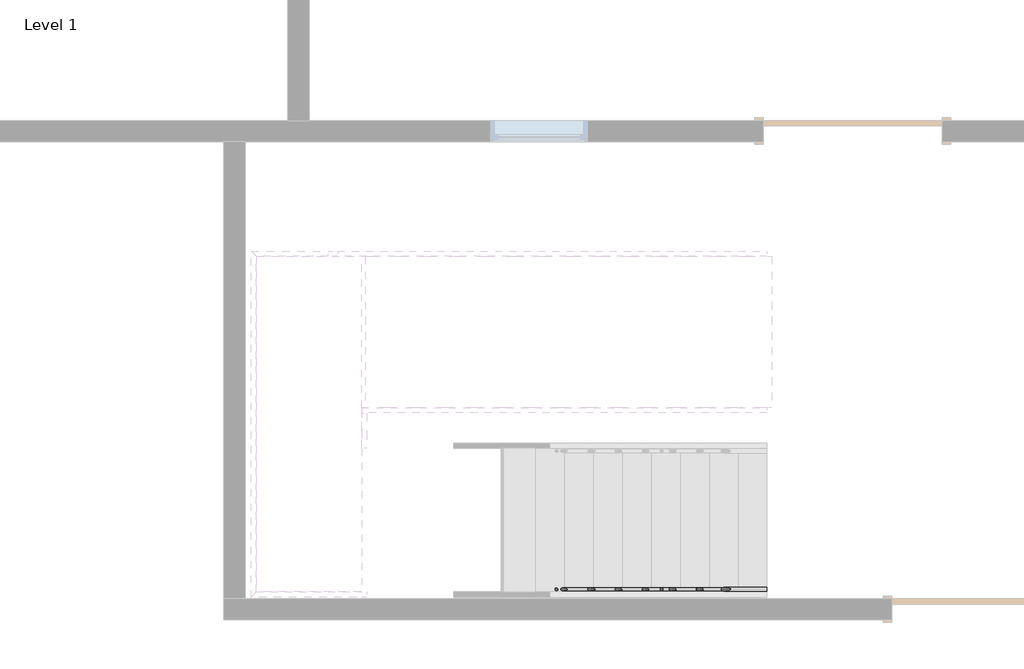
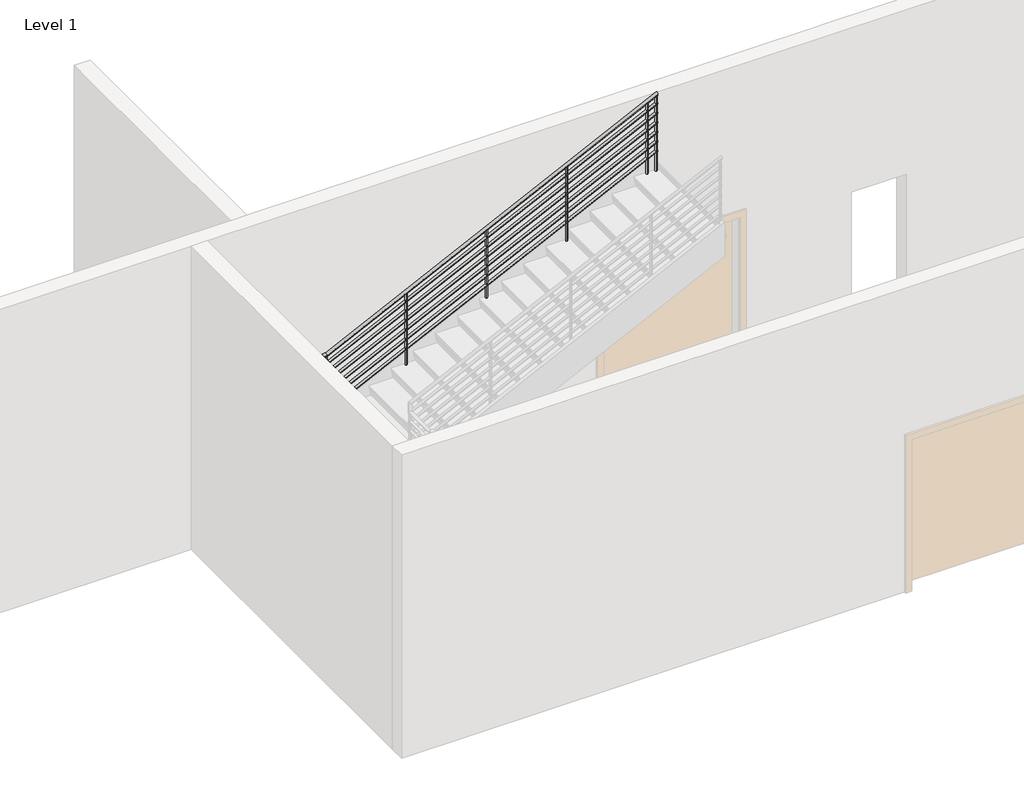
# One storey, part 3 of 4: 1 railing.
"""IFC4 building model written with IfcOpenShell, lengths in millimetres."""

from ifc_helpers import new_model, si_unit, point, frame, frame_2d, origin, place, context, project, spatial, circle_curve, ellipse_curve, trimmed, segment, composite_curve, outline, extrude, element, save
from ifc_brep_helpers import plane_surface, cylinder_surface, advanced_brep

model = new_model("IFC4")

# Units and contexts
model_context = context("Model", 3, world=origin())
ifc_project = project(units=[si_unit("LENGTHUNIT", "METRE", prefix="MILLI")], contexts=[model_context])

# Site, building, storey
site = spatial("IfcSite", under=ifc_project)
building = spatial("IfcBuilding", under=site)
storey = spatial("IfcBuildingStorey", under=building, Name="Level 1", Elevation=0.0)

# Railing
placement = place(None, origin())
element("IfcRailing", 1, ObjectType="900mm Pipe", at=placement, inside=storey, context=model_context, shape_type="SolidModel", body=[
    advanced_brep(
    [(3615.6033064, -1103.671626, 1011.1065202), (3615.6033064, -1143.671626, 1011.1065202), (-238.9894956, -1103.671626, 2880.0), (-238.9894956, -1143.671626, 2880.0), (-1189.0224748, -1103.671626, 2880.0), (-1229.0224748, -1143.671626, 2880.0), (-1189.0224748, 1993.0290713, 2880.0), (-1229.0224748, 2033.0290713, 2880.0), (-504.8038915, 1993.0290713, 2880.0), (-504.8038915, 2033.0290713, 2880.0), (3615.6033064, 1993.0290713, 4877.7731869), (3615.6033064, 2033.0290713, 4877.7731869)],
    [
        (0, 1, ellipse_curve(frame((3615.6033064, -1123.671626, 1011.1065202), z_axis=(1.0, 0.0, 0.0), x_axis=(0.0, 0.0, -1.0)), 22.2268131, 20.0)),
        (1, 0, ellipse_curve(frame((3615.6033064, -1123.671626, 1011.1065202), z_axis=(1.0, 0.0, 0.0), x_axis=(0.0, 0.0, -1.0)), 22.2268131, 20.0)),
        (0, 2),
        (2, 3, ellipse_curve(frame((-238.9894956, -1123.671626, 2880.0), z_axis=(0.9746317528164674, 0.0, -0.22381453572522994), x_axis=(-0.2238145357252298, 0.0, -0.9746317528164675)), 20.5205709, 20.0)),
        (3, 1),
        (3, 2, ellipse_curve(frame((-238.9894956, -1123.671626, 2880.0), z_axis=(0.9746317528164674, 0.0, -0.22381453572522994), x_axis=(-0.2238145357252298, 0.0, -0.9746317528164675)), 20.5205709, 20.0)),
        (2, 4),
        (4, 5, ellipse_curve(frame((-1209.0224748, -1123.671626, 2880.0), z_axis=(0.7071067811865449, -0.7071067811865501, 0.0), x_axis=(0.7071067811865501, 0.7071067811865449, 0.0)), 28.2842712, 20.0)),
        (5, 3),
        (5, 4, ellipse_curve(frame((-1209.0224748, -1123.671626, 2880.0), z_axis=(0.7071067811865449, -0.7071067811865501, 0.0), x_axis=(0.7071067811865501, 0.7071067811865449, 0.0)), 28.2842712, 20.0)),
        (4, 6),
        (6, 7, ellipse_curve(frame((-1209.0224748, 2013.0290713, 2880.0), z_axis=(-0.70710678118655, -0.7071067811865449, 0.0), x_axis=(0.7071067811865448, -0.7071067811865501, 0.0)), 28.2842712, 20.0)),
        (7, 5),
        (7, 6, ellipse_curve(frame((-1209.0224748, 2013.0290713, 2880.0), z_axis=(-0.70710678118655, -0.7071067811865449, 0.0), x_axis=(0.7071067811865448, -0.7071067811865501, 0.0)), 28.2842712, 20.0)),
        (6, 8),
        (8, 9, ellipse_curve(frame((-504.8038915, 2013.0290713, 2880.0), z_axis=(-0.9746317528164674, 0.0, -0.22381453572522989), x_axis=(-0.22381453572523038, 0.0, 0.9746317528164674)), 20.5205709, 20.0)),
        (9, 7),
        (9, 8, ellipse_curve(frame((-504.8038915, 2013.0290713, 2880.0), z_axis=(-0.9746317528164674, 0.0, -0.22381453572522989), x_axis=(-0.22381453572523038, 0.0, 0.9746317528164674)), 20.5205709, 20.0)),
        (10, 11, ellipse_curve(frame((3615.6033064, 2013.0290713, 4877.7731869), z_axis=(1.0, 0.0, 0.0), x_axis=(0.0, 0.0, -1.0)), 22.2268131, 20.0)),
        (11, 10, ellipse_curve(frame((3615.6033064, 2013.0290713, 4877.7731869), z_axis=(1.0, 0.0, 0.0), x_axis=(0.0, 0.0, -1.0)), 22.2268131, 20.0)),
        (8, 10),
        (11, 9),
    ],
    [
        plane_surface(frame((3615.6033064, -1123.671626, 1033.3333333), z_axis=(1.0, 0.0, 0.0), x_axis=(0.0, -1.0, 0.0))),
        cylinder_surface(frame((3606.8778363, -1123.671626, 1015.3370512), z_axis=(0.8998141071961996, 0.0, -0.4362735065193695), x_axis=(0.0, -1.0, 0.0)), 20.0),
        cylinder_surface(frame((-234.3966936, -1123.671626, 2880.0), z_axis=(1.0, 0.0, 0.0), x_axis=(0.0, -1.0, 0.0)), 20.0),
        cylinder_surface(frame((-1209.0224748, -1123.671626, 2880.0), z_axis=(0.0, -1.0, 0.0), x_axis=(-1.0, 0.0, 0.0)), 20.0),
        cylinder_surface(frame((-1209.0224748, 2013.0290713, 2880.0), z_axis=(-1.0, 0.0, 0.0), x_axis=(0.0, 1.0, 0.0)), 20.0),
        plane_surface(frame((3615.6033064, 2013.0290713, 4900.0), z_axis=(1.0, 0.0, 0.0), x_axis=(0.0, 1.0, 0.0))),
        cylinder_surface(frame((-500.6712235, 2013.0290713, 2882.0037179), z_axis=(-0.8998141071961996, 0.0, -0.4362735065193694), x_axis=(0.0, 1.0, 0.0)), 20.0),
    ],
    [
        (0, [[1, 2]]),
        (1, [[-1, 3, 4, 5]]),
        (1, [[-2, -5, 6, -3]]),
        (2, [[-4, 7, 8, 9]]),
        (2, [[-6, -9, 10, -7]]),
        (3, [[-8, 11, 12, 13]]),
        (3, [[-10, -13, 14, -11]]),
        (4, [[-12, 15, 16, 17]]),
        (4, [[-14, -17, 18, -15]]),
        (5, [[19, 20]]),
        (6, [[-16, 21, -20, 22]]),
        (6, [[-18, -22, -19, -21]]),
    ],
),
    advanced_brep(
    [(3615.6033064, -1108.671626, 891.6632235), (3615.6033064, -1138.671626, 891.6632235), (-237.8412951, -1108.671626, 2760.0), (-237.8412951, -1138.671626, 2760.0), (-1194.0224748, -1108.671626, 2760.0), (-1224.0224748, -1138.671626, 2760.0), (-1194.0224748, 1998.0290713, 2760.0), (-1224.0224748, 2028.0290713, 2760.0), (-505.952092, 1998.0290713, 2760.0), (-505.952092, 2028.0290713, 2760.0), (3615.6033064, 1998.0290713, 4758.3298902), (3615.6033064, 2028.0290713, 4758.3298902)],
    [
        (0, 1, ellipse_curve(frame((3615.6033064, -1123.671626, 891.6632235), z_axis=(1.0, 0.0, 0.0), x_axis=(0.0, 0.0, -1.0)), 16.6701098, 15.0)),
        (1, 0, ellipse_curve(frame((3615.6033064, -1123.671626, 891.6632235), z_axis=(1.0, 0.0, 0.0), x_axis=(0.0, 0.0, -1.0)), 16.6701098, 15.0)),
        (0, 2),
        (2, 3, ellipse_curve(frame((-237.8412951, -1123.671626, 2760.0), z_axis=(0.9746317528164674, 0.0, -0.22381453572522994), x_axis=(-0.2238145357252298, 0.0, -0.9746317528164675)), 15.3904282, 15.0)),
        (3, 1),
        (3, 2, ellipse_curve(frame((-237.8412951, -1123.671626, 2760.0), z_axis=(0.9746317528164674, 0.0, -0.22381453572522994), x_axis=(-0.2238145357252298, 0.0, -0.9746317528164675)), 15.3904282, 15.0)),
        (2, 4),
        (4, 5, ellipse_curve(frame((-1209.0224748, -1123.671626, 2760.0), z_axis=(0.7071067811865449, -0.7071067811865501, 0.0), x_axis=(0.7071067811865501, 0.7071067811865449, 0.0)), 21.2132034, 15.0)),
        (5, 3),
        (5, 4, ellipse_curve(frame((-1209.0224748, -1123.671626, 2760.0), z_axis=(0.7071067811865449, -0.7071067811865501, 0.0), x_axis=(0.7071067811865501, 0.7071067811865449, 0.0)), 21.2132034, 15.0)),
        (4, 6),
        (6, 7, ellipse_curve(frame((-1209.0224748, 2013.0290713, 2760.0), z_axis=(-0.70710678118655, -0.7071067811865449, 0.0), x_axis=(0.7071067811865448, -0.7071067811865501, 0.0)), 21.2132034, 15.0)),
        (7, 5),
        (7, 6, ellipse_curve(frame((-1209.0224748, 2013.0290713, 2760.0), z_axis=(-0.70710678118655, -0.7071067811865449, 0.0), x_axis=(0.7071067811865448, -0.7071067811865501, 0.0)), 21.2132034, 15.0)),
        (6, 8),
        (8, 9, ellipse_curve(frame((-505.952092, 2013.0290713, 2760.0), z_axis=(-0.9746317528164674, 0.0, -0.22381453572522989), x_axis=(-0.22381453572523038, 0.0, 0.9746317528164674)), 15.3904282, 15.0)),
        (9, 7),
        (9, 8, ellipse_curve(frame((-505.952092, 2013.0290713, 2760.0), z_axis=(-0.9746317528164674, 0.0, -0.22381453572522989), x_axis=(-0.22381453572523038, 0.0, 0.9746317528164674)), 15.3904282, 15.0)),
        (10, 11, ellipse_curve(frame((3615.6033064, 2013.0290713, 4758.3298902), z_axis=(1.0, 0.0, 0.0), x_axis=(0.0, 0.0, -1.0)), 16.6701098, 15.0)),
        (11, 10, ellipse_curve(frame((3615.6033064, 2013.0290713, 4758.3298902), z_axis=(1.0, 0.0, 0.0), x_axis=(0.0, 0.0, -1.0)), 16.6701098, 15.0)),
        (8, 10),
        (11, 9),
    ],
    [
        plane_surface(frame((3615.6033064, -1123.671626, 908.3333333), z_axis=(1.0, 0.0, 0.0), x_axis=(0.0, -1.0, 0.0))),
        cylinder_surface(frame((3609.0592038, -1123.671626, 894.8361217), z_axis=(0.8998141071961996, 0.0, -0.4362735065193695), x_axis=(0.0, -1.0, 0.0)), 15.0),
        cylinder_surface(frame((-234.3966936, -1123.671626, 2760.0), z_axis=(1.0, 0.0, 0.0), x_axis=(0.0, -1.0, 0.0)), 15.0),
        cylinder_surface(frame((-1209.0224748, -1123.671626, 2760.0), z_axis=(0.0, -1.0, 0.0), x_axis=(-1.0, 0.0, 0.0)), 15.0),
        cylinder_surface(frame((-1209.0224748, 2013.0290713, 2760.0), z_axis=(-1.0, 0.0, 0.0), x_axis=(0.0, 1.0, 0.0)), 15.0),
        plane_surface(frame((3615.6033064, 2013.0290713, 4775.0), z_axis=(1.0, 0.0, 0.0), x_axis=(0.0, 1.0, 0.0))),
        cylinder_surface(frame((-502.852591, 2013.0290713, 2761.5027884), z_axis=(-0.8998141071961996, 0.0, -0.4362735065193694), x_axis=(0.0, 1.0, 0.0)), 15.0),
    ],
    [
        (0, [[1, 2]]),
        (1, [[-1, 3, 4, 5]]),
        (1, [[-2, -5, 6, -3]]),
        (2, [[-4, 7, 8, 9]]),
        (2, [[-6, -9, 10, -7]]),
        (3, [[-8, 11, 12, 13]]),
        (3, [[-10, -13, 14, -11]]),
        (4, [[-12, 15, 16, 17]]),
        (4, [[-14, -17, 18, -15]]),
        (5, [[19, 20]]),
        (6, [[-16, 21, -20, 22]]),
        (6, [[-18, -22, -19, -21]]),
    ],
),
    advanced_brep(
    [(3615.6033064, -1108.671626, 766.6632235), (3615.6033064, -1138.671626, 766.6632235), (-237.8412951, -1108.671626, 2635.0), (-237.8412951, -1138.671626, 2635.0), (-1194.0224748, -1108.671626, 2635.0), (-1224.0224748, -1138.671626, 2635.0), (-1194.0224748, 1998.0290713, 2635.0), (-1224.0224748, 2028.0290713, 2635.0), (-505.952092, 1998.0290713, 2635.0), (-505.952092, 2028.0290713, 2635.0), (3615.6033064, 1998.0290713, 4633.3298902), (3615.6033064, 2028.0290713, 4633.3298902)],
    [
        (0, 1, ellipse_curve(frame((3615.6033064, -1123.671626, 766.6632235), z_axis=(1.0, 0.0, 0.0), x_axis=(0.0, 0.0, -1.0)), 16.6701098, 15.0)),
        (1, 0, ellipse_curve(frame((3615.6033064, -1123.671626, 766.6632235), z_axis=(1.0, 0.0, 0.0), x_axis=(0.0, 0.0, -1.0)), 16.6701098, 15.0)),
        (0, 2),
        (2, 3, ellipse_curve(frame((-237.8412951, -1123.671626, 2635.0), z_axis=(0.9746317528164674, 0.0, -0.22381453572522994), x_axis=(-0.2238145357252298, 0.0, -0.9746317528164675)), 15.3904282, 15.0)),
        (3, 1),
        (3, 2, ellipse_curve(frame((-237.8412951, -1123.671626, 2635.0), z_axis=(0.9746317528164674, 0.0, -0.22381453572522994), x_axis=(-0.2238145357252298, 0.0, -0.9746317528164675)), 15.3904282, 15.0)),
        (2, 4),
        (4, 5, ellipse_curve(frame((-1209.0224748, -1123.671626, 2635.0), z_axis=(0.7071067811865449, -0.7071067811865501, 0.0), x_axis=(0.7071067811865501, 0.7071067811865449, 0.0)), 21.2132034, 15.0)),
        (5, 3),
        (5, 4, ellipse_curve(frame((-1209.0224748, -1123.671626, 2635.0), z_axis=(0.7071067811865449, -0.7071067811865501, 0.0), x_axis=(0.7071067811865501, 0.7071067811865449, 0.0)), 21.2132034, 15.0)),
        (4, 6),
        (6, 7, ellipse_curve(frame((-1209.0224748, 2013.0290713, 2635.0), z_axis=(-0.70710678118655, -0.7071067811865449, 0.0), x_axis=(0.7071067811865448, -0.7071067811865501, 0.0)), 21.2132034, 15.0)),
        (7, 5),
        (7, 6, ellipse_curve(frame((-1209.0224748, 2013.0290713, 2635.0), z_axis=(-0.70710678118655, -0.7071067811865449, 0.0), x_axis=(0.7071067811865448, -0.7071067811865501, 0.0)), 21.2132034, 15.0)),
        (6, 8),
        (8, 9, ellipse_curve(frame((-505.952092, 2013.0290713, 2635.0), z_axis=(-0.9746317528164674, 0.0, -0.22381453572522989), x_axis=(-0.22381453572523038, 0.0, 0.9746317528164674)), 15.3904282, 15.0)),
        (9, 7),
        (9, 8, ellipse_curve(frame((-505.952092, 2013.0290713, 2635.0), z_axis=(-0.9746317528164674, 0.0, -0.22381453572522989), x_axis=(-0.22381453572523038, 0.0, 0.9746317528164674)), 15.3904282, 15.0)),
        (10, 11, ellipse_curve(frame((3615.6033064, 2013.0290713, 4633.3298902), z_axis=(1.0, 0.0, 0.0), x_axis=(0.0, 0.0, -1.0)), 16.6701098, 15.0)),
        (11, 10, ellipse_curve(frame((3615.6033064, 2013.0290713, 4633.3298902), z_axis=(1.0, 0.0, 0.0), x_axis=(0.0, 0.0, -1.0)), 16.6701098, 15.0)),
        (8, 10),
        (11, 9),
    ],
    [
        plane_surface(frame((3615.6033064, -1123.671626, 783.3333333), z_axis=(1.0, 0.0, 0.0), x_axis=(0.0, -1.0, 0.0))),
        cylinder_surface(frame((3609.0592038, -1123.671626, 769.8361217), z_axis=(0.8998141071961996, 0.0, -0.4362735065193695), x_axis=(0.0, -1.0, 0.0)), 15.0),
        cylinder_surface(frame((-234.3966936, -1123.671626, 2635.0), z_axis=(1.0, 0.0, 0.0), x_axis=(0.0, -1.0, 0.0)), 15.0),
        cylinder_surface(frame((-1209.0224748, -1123.671626, 2635.0), z_axis=(0.0, -1.0, 0.0), x_axis=(-1.0, 0.0, 0.0)), 15.0),
        cylinder_surface(frame((-1209.0224748, 2013.0290713, 2635.0), z_axis=(-1.0, 0.0, 0.0), x_axis=(0.0, 1.0, 0.0)), 15.0),
        plane_surface(frame((3615.6033064, 2013.0290713, 4650.0), z_axis=(1.0, 0.0, 0.0), x_axis=(0.0, 1.0, 0.0))),
        cylinder_surface(frame((-502.852591, 2013.0290713, 2636.5027884), z_axis=(-0.8998141071961996, 0.0, -0.4362735065193694), x_axis=(0.0, 1.0, 0.0)), 15.0),
    ],
    [
        (0, [[1, 2]]),
        (1, [[-1, 3, 4, 5]]),
        (1, [[-2, -5, 6, -3]]),
        (2, [[-4, 7, 8, 9]]),
        (2, [[-6, -9, 10, -7]]),
        (3, [[-8, 11, 12, 13]]),
        (3, [[-10, -13, 14, -11]]),
        (4, [[-12, 15, 16, 17]]),
        (4, [[-14, -17, 18, -15]]),
        (5, [[19, 20]]),
        (6, [[-16, 21, -20, 22]]),
        (6, [[-18, -22, -19, -21]]),
    ],
),
    advanced_brep(
    [(3615.6033064, -1108.671626, 641.6632235), (3615.6033064, -1138.671626, 641.6632235), (-237.8412951, -1108.671626, 2510.0), (-237.8412951, -1138.671626, 2510.0), (-1194.0224748, -1108.671626, 2510.0), (-1224.0224748, -1138.671626, 2510.0), (-1194.0224748, 1998.0290713, 2510.0), (-1224.0224748, 2028.0290713, 2510.0), (-505.952092, 1998.0290713, 2510.0), (-505.952092, 2028.0290713, 2510.0), (3615.6033064, 1998.0290713, 4508.3298902), (3615.6033064, 2028.0290713, 4508.3298902)],
    [
        (0, 1, ellipse_curve(frame((3615.6033064, -1123.671626, 641.6632235), z_axis=(1.0, 0.0, 0.0), x_axis=(0.0, 0.0, -1.0)), 16.6701098, 15.0)),
        (1, 0, ellipse_curve(frame((3615.6033064, -1123.671626, 641.6632235), z_axis=(1.0, 0.0, 0.0), x_axis=(0.0, 0.0, -1.0)), 16.6701098, 15.0)),
        (0, 2),
        (2, 3, ellipse_curve(frame((-237.8412951, -1123.671626, 2510.0), z_axis=(0.9746317528164674, 0.0, -0.2238145357252299), x_axis=(-0.22381453572522944, 0.0, -0.9746317528164676)), 15.3904282, 15.0)),
        (3, 1),
        (3, 2, ellipse_curve(frame((-237.8412951, -1123.671626, 2510.0), z_axis=(0.9746317528164674, 0.0, -0.2238145357252299), x_axis=(-0.22381453572522944, 0.0, -0.9746317528164676)), 15.3904282, 15.0)),
        (2, 4),
        (4, 5, ellipse_curve(frame((-1209.0224748, -1123.671626, 2510.0), z_axis=(0.7071067811865449, -0.7071067811865501, 0.0), x_axis=(0.7071067811865501, 0.7071067811865449, 0.0)), 21.2132034, 15.0)),
        (5, 3),
        (5, 4, ellipse_curve(frame((-1209.0224748, -1123.671626, 2510.0), z_axis=(0.7071067811865449, -0.7071067811865501, 0.0), x_axis=(0.7071067811865501, 0.7071067811865449, 0.0)), 21.2132034, 15.0)),
        (4, 6),
        (6, 7, ellipse_curve(frame((-1209.0224748, 2013.0290713, 2510.0), z_axis=(-0.70710678118655, -0.7071067811865449, 0.0), x_axis=(0.7071067811865448, -0.7071067811865501, 0.0)), 21.2132034, 15.0)),
        (7, 5),
        (7, 6, ellipse_curve(frame((-1209.0224748, 2013.0290713, 2510.0), z_axis=(-0.70710678118655, -0.7071067811865449, 0.0), x_axis=(0.7071067811865448, -0.7071067811865501, 0.0)), 21.2132034, 15.0)),
        (6, 8),
        (8, 9, ellipse_curve(frame((-505.952092, 2013.0290713, 2510.0), z_axis=(-0.9746317528164674, 0.0, -0.22381453572522994), x_axis=(-0.22381453572523038, 0.0, 0.9746317528164674)), 15.3904282, 15.0)),
        (9, 7),
        (9, 8, ellipse_curve(frame((-505.952092, 2013.0290713, 2510.0), z_axis=(-0.9746317528164674, 0.0, -0.22381453572522994), x_axis=(-0.22381453572523038, 0.0, 0.9746317528164674)), 15.3904282, 15.0)),
        (10, 11, ellipse_curve(frame((3615.6033064, 2013.0290713, 4508.3298902), z_axis=(1.0, 0.0, 0.0), x_axis=(0.0, 0.0, -1.0)), 16.6701098, 15.0)),
        (11, 10, ellipse_curve(frame((3615.6033064, 2013.0290713, 4508.3298902), z_axis=(1.0, 0.0, 0.0), x_axis=(0.0, 0.0, -1.0)), 16.6701098, 15.0)),
        (8, 10),
        (11, 9),
    ],
    [
        plane_surface(frame((3615.6033064, -1123.671626, 658.3333333), z_axis=(1.0, 0.0, 0.0), x_axis=(0.0, -1.0, 0.0))),
        cylinder_surface(frame((3609.0592038, -1123.671626, 644.8361217), z_axis=(0.8998141071961997, 0.0, -0.4362735065193694), x_axis=(0.0, -1.0, 0.0)), 15.0),
        cylinder_surface(frame((-234.3966936, -1123.671626, 2510.0), z_axis=(1.0, 0.0, 0.0), x_axis=(0.0, -1.0, 0.0)), 15.0),
        cylinder_surface(frame((-1209.0224748, -1123.671626, 2510.0), z_axis=(0.0, -1.0, 0.0), x_axis=(-1.0, 0.0, 0.0)), 15.0),
        cylinder_surface(frame((-1209.0224748, 2013.0290713, 2510.0), z_axis=(-1.0, 0.0, 0.0), x_axis=(0.0, 1.0, 0.0)), 15.0),
        plane_surface(frame((3615.6033064, 2013.0290713, 4525.0), z_axis=(1.0, 0.0, 0.0), x_axis=(0.0, 1.0, 0.0))),
        cylinder_surface(frame((-502.852591, 2013.0290713, 2511.5027884), z_axis=(-0.8998141071961996, 0.0, -0.43627350651936947), x_axis=(0.0, 1.0, 0.0)), 15.0),
    ],
    [
        (0, [[1, 2]]),
        (1, [[-1, 3, 4, 5]]),
        (1, [[-2, -5, 6, -3]]),
        (2, [[-4, 7, 8, 9]]),
        (2, [[-6, -9, 10, -7]]),
        (3, [[-8, 11, 12, 13]]),
        (3, [[-10, -13, 14, -11]]),
        (4, [[-12, 15, 16, 17]]),
        (4, [[-14, -17, 18, -15]]),
        (5, [[19, 20]]),
        (6, [[-16, 21, -20, 22]]),
        (6, [[-18, -22, -19, -21]]),
    ],
),
    advanced_brep(
    [(3615.6033064, -1108.671626, 516.6632235), (3615.6033064, -1138.671626, 516.6632235), (-237.8412951, -1108.671626, 2385.0), (-237.8412951, -1138.671626, 2385.0), (-1194.0224748, -1108.671626, 2385.0), (-1224.0224748, -1138.671626, 2385.0), (-1194.0224748, 1998.0290713, 2385.0), (-1224.0224748, 2028.0290713, 2385.0), (-505.952092, 1998.0290713, 2385.0), (-505.952092, 2028.0290713, 2385.0), (3615.6033064, 1998.0290713, 4383.3298902), (3615.6033064, 2028.0290713, 4383.3298902)],
    [
        (0, 1, ellipse_curve(frame((3615.6033064, -1123.671626, 516.6632235), z_axis=(1.0, 0.0, 0.0), x_axis=(0.0, 0.0, -1.0)), 16.6701098, 15.0)),
        (1, 0, ellipse_curve(frame((3615.6033064, -1123.671626, 516.6632235), z_axis=(1.0, 0.0, 0.0), x_axis=(0.0, 0.0, -1.0)), 16.6701098, 15.0)),
        (0, 2),
        (2, 3, ellipse_curve(frame((-237.8412951, -1123.671626, 2385.0), z_axis=(0.9746317528164674, 0.0, -0.22381453572522994), x_axis=(-0.2238145357252298, 0.0, -0.9746317528164675)), 15.3904282, 15.0)),
        (3, 1),
        (3, 2, ellipse_curve(frame((-237.8412951, -1123.671626, 2385.0), z_axis=(0.9746317528164674, 0.0, -0.22381453572522994), x_axis=(-0.2238145357252298, 0.0, -0.9746317528164675)), 15.3904282, 15.0)),
        (2, 4),
        (4, 5, ellipse_curve(frame((-1209.0224748, -1123.671626, 2385.0), z_axis=(0.7071067811865449, -0.7071067811865501, 0.0), x_axis=(0.7071067811865501, 0.7071067811865449, 0.0)), 21.2132034, 15.0)),
        (5, 3),
        (5, 4, ellipse_curve(frame((-1209.0224748, -1123.671626, 2385.0), z_axis=(0.7071067811865449, -0.7071067811865501, 0.0), x_axis=(0.7071067811865501, 0.7071067811865449, 0.0)), 21.2132034, 15.0)),
        (4, 6),
        (6, 7, ellipse_curve(frame((-1209.0224748, 2013.0290713, 2385.0), z_axis=(-0.70710678118655, -0.7071067811865449, 0.0), x_axis=(0.7071067811865448, -0.7071067811865501, 0.0)), 21.2132034, 15.0)),
        (7, 5),
        (7, 6, ellipse_curve(frame((-1209.0224748, 2013.0290713, 2385.0), z_axis=(-0.70710678118655, -0.7071067811865449, 0.0), x_axis=(0.7071067811865448, -0.7071067811865501, 0.0)), 21.2132034, 15.0)),
        (6, 8),
        (8, 9, ellipse_curve(frame((-505.952092, 2013.0290713, 2385.0), z_axis=(-0.9746317528164674, 0.0, -0.22381453572522989), x_axis=(-0.22381453572523038, 0.0, 0.9746317528164674)), 15.3904282, 15.0)),
        (9, 7),
        (9, 8, ellipse_curve(frame((-505.952092, 2013.0290713, 2385.0), z_axis=(-0.9746317528164674, 0.0, -0.22381453572522989), x_axis=(-0.22381453572523038, 0.0, 0.9746317528164674)), 15.3904282, 15.0)),
        (10, 11, ellipse_curve(frame((3615.6033064, 2013.0290713, 4383.3298902), z_axis=(1.0, 0.0, 0.0), x_axis=(0.0, 0.0, -1.0)), 16.6701098, 15.0)),
        (11, 10, ellipse_curve(frame((3615.6033064, 2013.0290713, 4383.3298902), z_axis=(1.0, 0.0, 0.0), x_axis=(0.0, 0.0, -1.0)), 16.6701098, 15.0)),
        (8, 10),
        (11, 9),
    ],
    [
        plane_surface(frame((3615.6033064, -1123.671626, 533.3333333), z_axis=(1.0, 0.0, 0.0), x_axis=(0.0, -1.0, 0.0))),
        cylinder_surface(frame((3609.0592038, -1123.671626, 519.8361217), z_axis=(0.8998141071961996, 0.0, -0.4362735065193695), x_axis=(0.0, -1.0, 0.0)), 15.0),
        cylinder_surface(frame((-234.3966936, -1123.671626, 2385.0), z_axis=(1.0, 0.0, 0.0), x_axis=(0.0, -1.0, 0.0)), 15.0),
        cylinder_surface(frame((-1209.0224748, -1123.671626, 2385.0), z_axis=(0.0, -1.0, 0.0), x_axis=(-1.0, 0.0, 0.0)), 15.0),
        cylinder_surface(frame((-1209.0224748, 2013.0290713, 2385.0), z_axis=(-1.0, 0.0, 0.0), x_axis=(0.0, 1.0, 0.0)), 15.0),
        plane_surface(frame((3615.6033064, 2013.0290713, 4400.0), z_axis=(1.0, 0.0, 0.0), x_axis=(0.0, 1.0, 0.0))),
        cylinder_surface(frame((-502.852591, 2013.0290713, 2386.5027884), z_axis=(-0.8998141071961996, 0.0, -0.4362735065193694), x_axis=(0.0, 1.0, 0.0)), 15.0),
    ],
    [
        (0, [[1, 2]]),
        (1, [[-1, 3, 4, 5]]),
        (1, [[-2, -5, 6, -3]]),
        (2, [[-4, 7, 8, 9]]),
        (2, [[-6, -9, 10, -7]]),
        (3, [[-8, 11, 12, 13]]),
        (3, [[-10, -13, 14, -11]]),
        (4, [[-12, 15, 16, 17]]),
        (4, [[-14, -17, 18, -15]]),
        (5, [[19, 20]]),
        (6, [[-16, 21, -20, 22]]),
        (6, [[-18, -22, -19, -21]]),
    ],
),
    advanced_brep(
    [(3615.6033064, -1108.671626, 391.6632235), (3615.6033064, -1138.671626, 391.6632235), (-237.8412951, -1108.671626, 2260.0), (-237.8412951, -1138.671626, 2260.0), (-1194.0224748, -1108.671626, 2260.0), (-1224.0224748, -1138.671626, 2260.0), (-1194.0224748, 1998.0290713, 2260.0), (-1224.0224748, 2028.0290713, 2260.0), (-505.952092, 1998.0290713, 2260.0), (-505.952092, 2028.0290713, 2260.0), (3615.6033064, 1998.0290713, 4258.3298902), (3615.6033064, 2028.0290713, 4258.3298902)],
    [
        (0, 1, ellipse_curve(frame((3615.6033064, -1123.671626, 391.6632235), z_axis=(1.0, 0.0, 0.0), x_axis=(0.0, 0.0, -1.0)), 16.6701098, 15.0)),
        (1, 0, ellipse_curve(frame((3615.6033064, -1123.671626, 391.6632235), z_axis=(1.0, 0.0, 0.0), x_axis=(0.0, 0.0, -1.0)), 16.6701098, 15.0)),
        (0, 2),
        (2, 3, ellipse_curve(frame((-237.8412951, -1123.671626, 2260.0), z_axis=(0.9746317528164674, 0.0, -0.22381453572522994), x_axis=(-0.2238145357252298, 0.0, -0.9746317528164675)), 15.3904282, 15.0)),
        (3, 1),
        (3, 2, ellipse_curve(frame((-237.8412951, -1123.671626, 2260.0), z_axis=(0.9746317528164674, 0.0, -0.22381453572522994), x_axis=(-0.2238145357252298, 0.0, -0.9746317528164675)), 15.3904282, 15.0)),
        (2, 4),
        (4, 5, ellipse_curve(frame((-1209.0224748, -1123.671626, 2260.0), z_axis=(0.7071067811865449, -0.7071067811865501, 0.0), x_axis=(0.7071067811865501, 0.7071067811865449, 0.0)), 21.2132034, 15.0)),
        (5, 3),
        (5, 4, ellipse_curve(frame((-1209.0224748, -1123.671626, 2260.0), z_axis=(0.7071067811865449, -0.7071067811865501, 0.0), x_axis=(0.7071067811865501, 0.7071067811865449, 0.0)), 21.2132034, 15.0)),
        (4, 6),
        (6, 7, ellipse_curve(frame((-1209.0224748, 2013.0290713, 2260.0), z_axis=(-0.70710678118655, -0.7071067811865449, 0.0), x_axis=(0.7071067811865448, -0.7071067811865501, 0.0)), 21.2132034, 15.0)),
        (7, 5),
        (7, 6, ellipse_curve(frame((-1209.0224748, 2013.0290713, 2260.0), z_axis=(-0.70710678118655, -0.7071067811865449, 0.0), x_axis=(0.7071067811865448, -0.7071067811865501, 0.0)), 21.2132034, 15.0)),
        (6, 8),
        (8, 9, ellipse_curve(frame((-505.952092, 2013.0290713, 2260.0), z_axis=(-0.9746317528164674, 0.0, -0.2238145357252299), x_axis=(-0.22381453572523033, 0.0, 0.9746317528164674)), 15.3904282, 15.0)),
        (9, 7),
        (9, 8, ellipse_curve(frame((-505.952092, 2013.0290713, 2260.0), z_axis=(-0.9746317528164674, 0.0, -0.2238145357252299), x_axis=(-0.22381453572523033, 0.0, 0.9746317528164674)), 15.3904282, 15.0)),
        (10, 11, ellipse_curve(frame((3615.6033064, 2013.0290713, 4258.3298902), z_axis=(1.0, 0.0, 0.0), x_axis=(0.0, 0.0, -1.0)), 16.6701098, 15.0)),
        (11, 10, ellipse_curve(frame((3615.6033064, 2013.0290713, 4258.3298902), z_axis=(1.0, 0.0, 0.0), x_axis=(0.0, 0.0, -1.0)), 16.6701098, 15.0)),
        (8, 10),
        (11, 9),
    ],
    [
        plane_surface(frame((3615.6033064, -1123.671626, 408.3333333), z_axis=(1.0, 0.0, 0.0), x_axis=(0.0, -1.0, 0.0))),
        cylinder_surface(frame((3609.0592038, -1123.671626, 394.8361217), z_axis=(0.8998141071961996, 0.0, -0.4362735065193695), x_axis=(0.0, -1.0, 0.0)), 15.0),
        cylinder_surface(frame((-234.3966936, -1123.671626, 2260.0), z_axis=(1.0, 0.0, 0.0), x_axis=(0.0, -1.0, 0.0)), 15.0),
        cylinder_surface(frame((-1209.0224748, -1123.671626, 2260.0), z_axis=(0.0, -1.0, 0.0), x_axis=(-1.0, 0.0, 0.0)), 15.0),
        cylinder_surface(frame((-1209.0224748, 2013.0290713, 2260.0), z_axis=(-1.0, 0.0, 0.0), x_axis=(0.0, 1.0, 0.0)), 15.0),
        plane_surface(frame((3615.6033064, 2013.0290713, 4275.0), z_axis=(1.0, 0.0, 0.0), x_axis=(0.0, 1.0, 0.0))),
        cylinder_surface(frame((-502.852591, 2013.0290713, 2261.5027884), z_axis=(-0.8998141071961996, 0.0, -0.43627350651936947), x_axis=(0.0, 1.0, 0.0)), 15.0),
    ],
    [
        (0, [[1, 2]]),
        (1, [[-1, 3, 4, 5]]),
        (1, [[-2, -5, 6, -3]]),
        (2, [[-4, 7, 8, 9]]),
        (2, [[-6, -9, 10, -7]]),
        (3, [[-8, 11, 12, 13]]),
        (3, [[-10, -13, 14, -11]]),
        (4, [[-12, 15, 16, 17]]),
        (4, [[-14, -17, 18, -15]]),
        (5, [[19, 20]]),
        (6, [[-16, 21, -20, 22]]),
        (6, [[-18, -22, -19, -21]]),
    ],
),
    advanced_brep(
    [(3615.6033064, -1108.671626, 266.6632235), (3615.6033064, -1138.671626, 266.6632235), (-237.8412951, -1108.671626, 2135.0), (-237.8412951, -1138.671626, 2135.0), (-1194.0224748, -1108.671626, 2135.0), (-1224.0224748, -1138.671626, 2135.0), (-1194.0224748, 1998.0290713, 2135.0), (-1224.0224748, 2028.0290713, 2135.0), (-505.952092, 1998.0290713, 2135.0), (-505.952092, 2028.0290713, 2135.0), (3615.6033064, 1998.0290713, 4133.3298902), (3615.6033064, 2028.0290713, 4133.3298902)],
    [
        (0, 1, ellipse_curve(frame((3615.6033064, -1123.671626, 266.6632235), z_axis=(1.0, 0.0, 0.0), x_axis=(0.0, 0.0, -1.0)), 16.6701098, 15.0)),
        (1, 0, ellipse_curve(frame((3615.6033064, -1123.671626, 266.6632235), z_axis=(1.0, 0.0, 0.0), x_axis=(0.0, 0.0, -1.0)), 16.6701098, 15.0)),
        (0, 2),
        (2, 3, ellipse_curve(frame((-237.8412951, -1123.671626, 2135.0), z_axis=(0.9746317528164674, 0.0, -0.22381453572522994), x_axis=(-0.2238145357252298, 0.0, -0.9746317528164675)), 15.3904282, 15.0)),
        (3, 1),
        (3, 2, ellipse_curve(frame((-237.8412951, -1123.671626, 2135.0), z_axis=(0.9746317528164674, 0.0, -0.22381453572522994), x_axis=(-0.2238145357252298, 0.0, -0.9746317528164675)), 15.3904282, 15.0)),
        (2, 4),
        (4, 5, ellipse_curve(frame((-1209.0224748, -1123.671626, 2135.0), z_axis=(0.7071067811865449, -0.7071067811865501, 0.0), x_axis=(0.7071067811865501, 0.7071067811865449, 0.0)), 21.2132034, 15.0)),
        (5, 3),
        (5, 4, ellipse_curve(frame((-1209.0224748, -1123.671626, 2135.0), z_axis=(0.7071067811865449, -0.7071067811865501, 0.0), x_axis=(0.7071067811865501, 0.7071067811865449, 0.0)), 21.2132034, 15.0)),
        (4, 6),
        (6, 7, ellipse_curve(frame((-1209.0224748, 2013.0290713, 2135.0), z_axis=(-0.70710678118655, -0.7071067811865449, 0.0), x_axis=(0.7071067811865448, -0.7071067811865501, 0.0)), 21.2132034, 15.0)),
        (7, 5),
        (7, 6, ellipse_curve(frame((-1209.0224748, 2013.0290713, 2135.0), z_axis=(-0.70710678118655, -0.7071067811865449, 0.0), x_axis=(0.7071067811865448, -0.7071067811865501, 0.0)), 21.2132034, 15.0)),
        (6, 8),
        (8, 9, ellipse_curve(frame((-505.952092, 2013.0290713, 2135.0), z_axis=(-0.9746317528164674, 0.0, -0.22381453572522989), x_axis=(-0.22381453572523038, 0.0, 0.9746317528164674)), 15.3904282, 15.0)),
        (9, 7),
        (9, 8, ellipse_curve(frame((-505.952092, 2013.0290713, 2135.0), z_axis=(-0.9746317528164674, 0.0, -0.22381453572522989), x_axis=(-0.22381453572523038, 0.0, 0.9746317528164674)), 15.3904282, 15.0)),
        (10, 11, ellipse_curve(frame((3615.6033064, 2013.0290713, 4133.3298902), z_axis=(1.0, 0.0, 0.0), x_axis=(0.0, 0.0, -1.0)), 16.6701098, 15.0)),
        (11, 10, ellipse_curve(frame((3615.6033064, 2013.0290713, 4133.3298902), z_axis=(1.0, 0.0, 0.0), x_axis=(0.0, 0.0, -1.0)), 16.6701098, 15.0)),
        (8, 10),
        (11, 9),
    ],
    [
        plane_surface(frame((3615.6033064, -1123.671626, 283.3333333), z_axis=(1.0, 0.0, 0.0), x_axis=(0.0, -1.0, 0.0))),
        cylinder_surface(frame((3609.0592038, -1123.671626, 269.8361217), z_axis=(0.8998141071961996, 0.0, -0.4362735065193695), x_axis=(0.0, -1.0, 0.0)), 15.0),
        cylinder_surface(frame((-234.3966936, -1123.671626, 2135.0), z_axis=(1.0, 0.0, 0.0), x_axis=(0.0, -1.0, 0.0)), 15.0),
        cylinder_surface(frame((-1209.0224748, -1123.671626, 2135.0), z_axis=(0.0, -1.0, 0.0), x_axis=(-1.0, 0.0, 0.0)), 15.0),
        cylinder_surface(frame((-1209.0224748, 2013.0290713, 2135.0), z_axis=(-1.0, 0.0, 0.0), x_axis=(0.0, 1.0, 0.0)), 15.0),
        plane_surface(frame((3615.6033064, 2013.0290713, 4150.0), z_axis=(1.0, 0.0, 0.0), x_axis=(0.0, 1.0, 0.0))),
        cylinder_surface(frame((-502.852591, 2013.0290713, 2136.5027884), z_axis=(-0.8998141071961996, 0.0, -0.4362735065193694), x_axis=(0.0, 1.0, 0.0)), 15.0),
    ],
    [
        (0, [[1, 2]]),
        (1, [[-1, 3, 4, 5]]),
        (1, [[-2, -5, 6, -3]]),
        (2, [[-4, 7, 8, 9]]),
        (2, [[-6, -9, 10, -7]]),
        (3, [[-8, 11, 12, 13]]),
        (3, [[-10, -13, 14, -11]]),
        (4, [[-12, 15, 16, 17]]),
        (4, [[-14, -17, 18, -15]]),
        (5, [[19, 20]]),
        (6, [[-16, 21, -20, 22]]),
        (6, [[-18, -22, -19, -21]]),
    ],
),
    advanced_brep(
    [(3490.6033064, 2025.5290713, 4794.9403132), (3490.6033064, 2000.5290713, 4794.9403132), (3490.6033064, 2000.5290713, 3866.6666667), (3490.6033064, 2025.5290713, 3866.6666667)],
    [
        (0, 1, ellipse_curve(frame((3490.6033064, 2013.0290713, 4794.9403132), z_axis=(0.43627350651937075, 0.0, -0.899814107196199), x_axis=(0.8998141071961991, 0.0, 0.43627350651937047)), 13.8917582, 12.5)),
        (1, 2),
        (2, 3, circle_curve(frame((3490.6033064, 2013.0290713, 3866.6666667), z_axis=(0.0, 0.0, 1.0), x_axis=(0.0, -1.0, 0.0)), 12.5)),
        (3, 0),
        (3, 2, circle_curve(frame((3490.6033064, 2013.0290713, 3866.6666667), z_axis=(0.0, 0.0, 1.0), x_axis=(0.0, -1.0, 0.0)), 12.5)),
        (1, 0, ellipse_curve(frame((3490.6033064, 2013.0290713, 4794.9403132), z_axis=(0.43627350651937075, 0.0, -0.899814107196199), x_axis=(0.8998141071961991, 0.0, 0.43627350651937047)), 13.8917582, 12.5)),
    ],
    [
        cylinder_surface(frame((3490.6033064, 2013.0290713, 3766.6666667), z_axis=(0.0, 0.0, 1.0), x_axis=(0.0, -1.0, 0.0)), 12.5),
        plane_surface(frame((3515.6033064, 1988.0290713, 4807.0615253), z_axis=(-0.43627350651937075, 0.0, 0.899814107196199), x_axis=(0.0, 1.0, 0.0))),
        plane_surface(frame((3465.6033064, 1988.0290713, 3866.6666667), z_axis=(0.0, 0.0, -1.0), x_axis=(0.0, 1.0, 0.0))),
    ],
    [
        (0, [[1, 2, 3, 4]]),
        (0, [[5, -2, 6, -4]]),
        (1, [[-6, -1]]),
        (2, [[-5, -3]]),
    ],
),
    advanced_brep(
    [(2490.6033064, 2025.5290713, 4310.0918283), (2490.6033064, 2000.5290713, 4310.0918283), (2490.6033064, 2000.5290713, 3333.3333333), (2490.6033064, 2025.5290713, 3333.3333333)],
    [
        (0, 1, ellipse_curve(frame((2490.6033064, 2013.0290713, 4310.0918283), z_axis=(0.43627350651937075, 0.0, -0.899814107196199), x_axis=(0.8998141071961991, 0.0, 0.43627350651937047)), 13.8917582, 12.5)),
        (1, 2),
        (2, 3, circle_curve(frame((2490.6033064, 2013.0290713, 3333.3333333), z_axis=(0.0, 0.0, 1.0), x_axis=(0.0, -1.0, 0.0)), 12.5)),
        (3, 0),
        (3, 2, circle_curve(frame((2490.6033064, 2013.0290713, 3333.3333333), z_axis=(0.0, 0.0, 1.0), x_axis=(0.0, -1.0, 0.0)), 12.5)),
        (1, 0, ellipse_curve(frame((2490.6033064, 2013.0290713, 4310.0918283), z_axis=(0.43627350651937075, 0.0, -0.899814107196199), x_axis=(0.8998141071961991, 0.0, 0.43627350651937047)), 13.8917582, 12.5)),
    ],
    [
        cylinder_surface(frame((2490.6033064, 2013.0290713, 3233.3333333), z_axis=(0.0, 0.0, 1.0), x_axis=(0.0, -1.0, 0.0)), 12.5),
        plane_surface(frame((2515.6033064, 1988.0290713, 4322.2130404), z_axis=(-0.43627350651937075, 0.0, 0.899814107196199), x_axis=(0.0, 1.0, 0.0))),
        plane_surface(frame((2465.6033064, 1988.0290713, 3333.3333333), z_axis=(0.0, 0.0, -1.0), x_axis=(0.0, 1.0, 0.0))),
    ],
    [
        (0, [[1, 2, 3, 4]]),
        (0, [[5, -2, 6, -4]]),
        (1, [[-6, -1]]),
        (2, [[-5, -3]]),
    ],
),
    advanced_brep(
    [(1490.6033064, 2025.5290713, 3825.2433435), (1490.6033064, 2000.5290713, 3825.2433435), (1490.6033064, 2000.5290713, 2933.3333333), (1490.6033064, 2025.5290713, 2933.3333333)],
    [
        (0, 1, ellipse_curve(frame((1490.6033064, 2013.0290713, 3825.2433435), z_axis=(0.43627350651937075, 0.0, -0.899814107196199), x_axis=(0.8998141071961991, 0.0, 0.43627350651937047)), 13.8917582, 12.5)),
        (1, 2),
        (2, 3, circle_curve(frame((1490.6033064, 2013.0290713, 2933.3333333), z_axis=(0.0, 0.0, 1.0), x_axis=(0.0, -1.0, 0.0)), 12.5)),
        (3, 0),
        (3, 2, circle_curve(frame((1490.6033064, 2013.0290713, 2933.3333333), z_axis=(0.0, 0.0, 1.0), x_axis=(0.0, -1.0, 0.0)), 12.5)),
        (1, 0, ellipse_curve(frame((1490.6033064, 2013.0290713, 3825.2433435), z_axis=(0.43627350651937075, 0.0, -0.899814107196199), x_axis=(0.8998141071961991, 0.0, 0.43627350651937047)), 13.8917582, 12.5)),
    ],
    [
        cylinder_surface(frame((1490.6033064, 2013.0290713, 2833.3333333), z_axis=(0.0, 0.0, 1.0), x_axis=(0.0, -1.0, 0.0)), 12.5),
        plane_surface(frame((1515.6033064, 1988.0290713, 3837.3645556), z_axis=(-0.43627350651937075, 0.0, 0.899814107196199), x_axis=(0.0, 1.0, 0.0))),
        plane_surface(frame((1465.6033064, 1988.0290713, 2933.3333333), z_axis=(0.0, 0.0, -1.0), x_axis=(0.0, 1.0, 0.0))),
    ],
    [
        (0, [[1, 2, 3, 4]]),
        (0, [[5, -2, 6, -4]]),
        (1, [[-6, -1]]),
        (2, [[-5, -3]]),
    ],
),
    advanced_brep(
    [(490.6033064, 2025.5290713, 3340.3948586), (490.6033064, 2000.5290713, 3340.3948586), (490.6033064, 2000.5290713, 2400.0), (490.6033064, 2025.5290713, 2400.0)],
    [
        (0, 1, ellipse_curve(frame((490.6033064, 2013.0290713, 3340.3948586), z_axis=(0.4362735065193688, 0.0, -0.8998141071961999), x_axis=(0.8998141071961999, 0.0, 0.4362735065193686)), 13.8917582, 12.5)),
        (1, 2),
        (2, 3, circle_curve(frame((490.6033064, 2013.0290713, 2400.0), z_axis=(0.0, 0.0, 1.0), x_axis=(0.0, -1.0, 0.0)), 12.5)),
        (3, 0),
        (3, 2, circle_curve(frame((490.6033064, 2013.0290713, 2400.0), z_axis=(0.0, 0.0, 1.0), x_axis=(0.0, -1.0, 0.0)), 12.5)),
        (1, 0, ellipse_curve(frame((490.6033064, 2013.0290713, 3340.3948586), z_axis=(0.4362735065193688, 0.0, -0.8998141071961999), x_axis=(0.8998141071961999, 0.0, 0.4362735065193686)), 13.8917582, 12.5)),
    ],
    [
        cylinder_surface(frame((490.6033064, 2013.0290713, 2300.0), z_axis=(0.0, 0.0, 1.0), x_axis=(0.0, -1.0, 0.0)), 12.5),
        plane_surface(frame((515.6033064, 1988.0290713, 3352.5160707), z_axis=(-0.4362735065193688, 0.0, 0.8998141071961999), x_axis=(0.0, 1.0, 0.0))),
        plane_surface(frame((465.6033064, 1988.0290713, 2400.0), z_axis=(0.0, 0.0, -1.0), x_axis=(0.0, 1.0, 0.0))),
    ],
    [
        (0, [[1, 2, 3, 4]]),
        (0, [[5, -2, 6, -4]]),
        (1, [[-6, -1]]),
        (2, [[-5, -3]]),
    ],
),
    extrude(outline(composite_curve([segment(trimmed(circle_curve(frame_2d((-1209.0224748, 1876.328374)), 12.5), [point((-1196.5224748, 1876.328374))], [point((-1221.5224748, 1876.328374))], False, "CARTESIAN"), True, "CONTINUOUS"), segment(trimmed(circle_curve(frame_2d((-1209.0224748, 1876.328374)), 12.5), [point((-1221.5224748, 1876.328374))], [point((-1196.5224748, 1876.328374))], False, "CARTESIAN"), True, "CONTINUOUS")], self_intersect=False)), frame((0.0, 0.0, 2000.0), z_axis=(0.0, 0.0, 1.0), x_axis=(1.0, 0.0, 0.0)), (0.0, 0.0, 1.0), 860.0),
    extrude(outline(composite_curve([segment(trimmed(circle_curve(frame_2d((-1209.0224748, 876.328374)), 12.5), [point((-1196.5224748, 876.328374))], [point((-1221.5224748, 876.328374))], False, "CARTESIAN"), True, "CONTINUOUS"), segment(trimmed(circle_curve(frame_2d((-1209.0224748, 876.328374)), 12.5), [point((-1221.5224748, 876.328374))], [point((-1196.5224748, 876.328374))], False, "CARTESIAN"), True, "CONTINUOUS")], self_intersect=False)), frame((0.0, 0.0, 2000.0), z_axis=(0.0, 0.0, 1.0), x_axis=(1.0, 0.0, 0.0)), (0.0, 0.0, 1.0), 860.0),
    extrude(outline(composite_curve([segment(trimmed(circle_curve(frame_2d((-1209.0224748, -123.671626)), 12.5), [point((-1196.5224748, -123.671626))], [point((-1221.5224748, -123.671626))], False, "CARTESIAN"), True, "CONTINUOUS"), segment(trimmed(circle_curve(frame_2d((-1209.0224748, -123.671626)), 12.5), [point((-1221.5224748, -123.671626))], [point((-1196.5224748, -123.671626))], False, "CARTESIAN"), True, "CONTINUOUS")], self_intersect=False)), frame((0.0, 0.0, 2000.0), z_axis=(0.0, 0.0, 1.0), x_axis=(1.0, 0.0, 0.0)), (0.0, 0.0, 1.0), 860.0),
    advanced_brep(
    [(615.6033064, -1136.171626, 2443.4251616), (615.6033064, -1111.171626, 2443.4251616), (615.6033064, -1111.171626, 1466.6666667), (615.6033064, -1136.171626, 1466.6666667)],
    [
        (0, 1, ellipse_curve(frame((615.6033064, -1123.671626, 2443.4251616), z_axis=(-0.43627350651937075, 0.0, -0.899814107196199), x_axis=(-0.8998141071961991, 0.0, 0.43627350651937047)), 13.8917582, 12.5)),
        (1, 2),
        (2, 3, circle_curve(frame((615.6033064, -1123.671626, 1466.6666667), z_axis=(0.0, 0.0, 1.0), x_axis=(0.0, 1.0, 0.0)), 12.5)),
        (3, 0),
        (3, 2, circle_curve(frame((615.6033064, -1123.671626, 1466.6666667), z_axis=(0.0, 0.0, 1.0), x_axis=(0.0, 1.0, 0.0)), 12.5)),
        (1, 0, ellipse_curve(frame((615.6033064, -1123.671626, 2443.4251616), z_axis=(-0.43627350651937075, 0.0, -0.899814107196199), x_axis=(-0.8998141071961991, 0.0, 0.43627350651937047)), 13.8917582, 12.5)),
    ],
    [
        cylinder_surface(frame((615.6033064, -1123.671626, 1366.6666667), z_axis=(0.0, 0.0, 1.0), x_axis=(0.0, 1.0, 0.0)), 12.5),
        plane_surface(frame((590.6033064, -1098.671626, 2455.5463738), z_axis=(0.43627350651937075, 0.0, 0.899814107196199), x_axis=(0.0, -1.0, 0.0))),
        plane_surface(frame((640.6033064, -1098.671626, 1466.6666667), z_axis=(0.0, 0.0, -1.0), x_axis=(0.0, -1.0, 0.0))),
    ],
    [
        (0, [[1, 2, 3, 4]]),
        (0, [[5, -2, 6, -4]]),
        (1, [[-6, -1]]),
        (2, [[-5, -3]]),
    ],
),
    advanced_brep(
    [(1615.6033064, -1136.171626, 1958.5766768), (1615.6033064, -1111.171626, 1958.5766768), (1615.6033064, -1111.171626, 1066.6666667), (1615.6033064, -1136.171626, 1066.6666667)],
    [
        (0, 1, ellipse_curve(frame((1615.6033064, -1123.671626, 1958.5766768), z_axis=(-0.43627350651937075, 0.0, -0.899814107196199), x_axis=(-0.8998141071961991, 0.0, 0.43627350651937047)), 13.8917582, 12.5)),
        (1, 2),
        (2, 3, circle_curve(frame((1615.6033064, -1123.671626, 1066.6666667), z_axis=(0.0, 0.0, 1.0), x_axis=(0.0, 1.0, 0.0)), 12.5)),
        (3, 0),
        (3, 2, circle_curve(frame((1615.6033064, -1123.671626, 1066.6666667), z_axis=(0.0, 0.0, 1.0), x_axis=(0.0, 1.0, 0.0)), 12.5)),
        (1, 0, ellipse_curve(frame((1615.6033064, -1123.671626, 1958.5766768), z_axis=(-0.43627350651937075, 0.0, -0.899814107196199), x_axis=(-0.8998141071961991, 0.0, 0.43627350651937047)), 13.8917582, 12.5)),
    ],
    [
        cylinder_surface(frame((1615.6033064, -1123.671626, 966.6666667), z_axis=(0.0, 0.0, 1.0), x_axis=(0.0, 1.0, 0.0)), 12.5),
        plane_surface(frame((1590.6033064, -1098.671626, 1970.6978889), z_axis=(0.43627350651937075, 0.0, 0.899814107196199), x_axis=(0.0, -1.0, 0.0))),
        plane_surface(frame((1640.6033064, -1098.671626, 1066.6666667), z_axis=(0.0, 0.0, -1.0), x_axis=(0.0, -1.0, 0.0))),
    ],
    [
        (0, [[1, 2, 3, 4]]),
        (0, [[5, -2, 6, -4]]),
        (1, [[-6, -1]]),
        (2, [[-5, -3]]),
    ],
),
    advanced_brep(
    [(2615.6033064, -1136.171626, 1473.7281919), (2615.6033064, -1111.171626, 1473.7281919), (2615.6033064, -1111.171626, 533.3333333), (2615.6033064, -1136.171626, 533.3333333)],
    [
        (0, 1, ellipse_curve(frame((2615.6033064, -1123.671626, 1473.7281919), z_axis=(-0.4362735065193688, 0.0, -0.8998141071961999), x_axis=(-0.8998141071961999, 0.0, 0.4362735065193686)), 13.8917582, 12.5)),
        (1, 2),
        (2, 3, circle_curve(frame((2615.6033064, -1123.671626, 533.3333333), z_axis=(0.0, 0.0, 1.0), x_axis=(0.0, 1.0, 0.0)), 12.5)),
        (3, 0),
        (3, 2, circle_curve(frame((2615.6033064, -1123.671626, 533.3333333), z_axis=(0.0, 0.0, 1.0), x_axis=(0.0, 1.0, 0.0)), 12.5)),
        (1, 0, ellipse_curve(frame((2615.6033064, -1123.671626, 1473.7281919), z_axis=(-0.4362735065193688, 0.0, -0.8998141071961999), x_axis=(-0.8998141071961999, 0.0, 0.4362735065193686)), 13.8917582, 12.5)),
    ],
    [
        cylinder_surface(frame((2615.6033064, -1123.671626, 433.3333333), z_axis=(0.0, 0.0, 1.0), x_axis=(0.0, 1.0, 0.0)), 12.5),
        plane_surface(frame((2590.6033064, -1098.671626, 1485.8494041), z_axis=(0.4362735065193688, 0.0, 0.8998141071961999), x_axis=(0.0, -1.0, 0.0))),
        plane_surface(frame((2640.6033064, -1098.671626, 533.3333333), z_axis=(0.0, 0.0, -1.0), x_axis=(0.0, -1.0, 0.0))),
    ],
    [
        (0, [[1, 2, 3, 4]]),
        (0, [[5, -2, 6, -4]]),
        (1, [[-6, -1]]),
        (2, [[-5, -3]]),
    ],
),
    extrude(outline(composite_curve([segment(trimmed(circle_curve(frame_2d((-509.3966936, 2013.0290713)), 12.5), [point((-509.3966936, 2000.5290713))], [point((-509.3966936, 2025.5290713))], False, "CARTESIAN"), True, "CONTINUOUS"), segment(trimmed(circle_curve(frame_2d((-509.3966936, 2013.0290713)), 12.5), [point((-509.3966936, 2025.5290713))], [point((-509.3966936, 2000.5290713))], False, "CARTESIAN"), True, "CONTINUOUS")], self_intersect=False)), frame((0.0, 0.0, 2000.0), z_axis=(0.0, 0.0, 1.0), x_axis=(1.0, 0.0, 0.0)), (0.0, 0.0, 1.0), 860.0),
    extrude(outline(composite_curve([segment(trimmed(circle_curve(frame_2d((-1209.0224748, 2013.0290713)), 12.5), [point((-1196.5224748, 2013.0290713))], [point((-1221.5224748, 2013.0290713))], False, "CARTESIAN"), True, "CONTINUOUS"), segment(trimmed(circle_curve(frame_2d((-1209.0224748, 2013.0290713)), 12.5), [point((-1221.5224748, 2013.0290713))], [point((-1196.5224748, 2013.0290713))], False, "CARTESIAN"), True, "CONTINUOUS")], self_intersect=False)), frame((0.0, 0.0, 2000.0), z_axis=(0.0, 0.0, 1.0), x_axis=(1.0, 0.0, 0.0)), (0.0, 0.0, 1.0), 860.0),
    extrude(outline(composite_curve([segment(trimmed(circle_curve(frame_2d((-1209.0224748, -1123.671626)), 12.5), [point((-1209.0224748, -1111.171626))], [point((-1209.0224748, -1136.171626))], False, "CARTESIAN"), True, "CONTINUOUS"), segment(trimmed(circle_curve(frame_2d((-1209.0224748, -1123.671626)), 12.5), [point((-1209.0224748, -1136.171626))], [point((-1209.0224748, -1111.171626))], False, "CARTESIAN"), True, "CONTINUOUS")], self_intersect=False)), frame((0.0, 0.0, 2000.0), z_axis=(0.0, 0.0, 1.0), x_axis=(1.0, 0.0, 0.0)), (0.0, 0.0, 1.0), 860.0),
    advanced_brep(
    [(-234.3966936, -1136.171626, 2855.5463738), (-234.3966936, -1111.171626, 2855.5463738), (-234.3966936, -1111.171626, 2000.0), (-234.3966936, -1136.171626, 2000.0)],
    [
        (0, 1, ellipse_curve(frame((-234.3966936, -1123.671626, 2855.5463738), z_axis=(-0.4362735065193688, 0.0, -0.8998141071961999), x_axis=(-0.8998141071961999, 0.0, 0.4362735065193686)), 13.8917582, 12.5)),
        (1, 2),
        (2, 3, circle_curve(frame((-234.3966936, -1123.671626, 2000.0), z_axis=(0.0, 0.0, 1.0), x_axis=(0.0, 1.0, 0.0)), 12.5)),
        (3, 0),
        (3, 2, circle_curve(frame((-234.3966936, -1123.671626, 2000.0), z_axis=(0.0, 0.0, 1.0), x_axis=(0.0, 1.0, 0.0)), 12.5)),
        (1, 0, ellipse_curve(frame((-234.3966936, -1123.671626, 2855.5463738), z_axis=(-0.4362735065193688, 0.0, -0.8998141071961999), x_axis=(-0.8998141071961999, 0.0, 0.4362735065193686)), 13.8917582, 12.5)),
    ],
    [
        cylinder_surface(frame((-234.3966936, -1123.671626, 1900.0), z_axis=(0.0, 0.0, 1.0), x_axis=(0.0, 1.0, 0.0)), 12.5),
        plane_surface(frame((-259.3966936, -1098.671626, 2867.6675859), z_axis=(0.4362735065193688, 0.0, 0.8998141071961999), x_axis=(0.0, -1.0, 0.0))),
        plane_surface(frame((-209.3966936, -1098.671626, 2000.0), z_axis=(0.0, 0.0, -1.0), x_axis=(0.0, -1.0, 0.0))),
    ],
    [
        (0, [[1, 2, 3, 4]]),
        (0, [[5, -2, 6, -4]]),
        (1, [[-6, -1]]),
        (2, [[-5, -3]]),
    ],
),
    advanced_brep(
    [(3603.1033064, 2025.5290713, 4849.4857677), (3603.1033064, 2000.5290713, 4849.4857677), (3603.1033064, 2000.5290713, 3866.6666667), (3603.1033064, 2025.5290713, 3866.6666667)],
    [
        (0, 1, ellipse_curve(frame((3603.1033064, 2013.0290713, 4849.4857677), z_axis=(0.4362735065193688, 0.0, -0.8998141071961999), x_axis=(0.8998141071961999, 0.0, 0.4362735065193686)), 13.8917582, 12.5)),
        (1, 2),
        (2, 3, circle_curve(frame((3603.1033064, 2013.0290713, 3866.6666667), z_axis=(0.0, 0.0, 1.0), x_axis=(0.0, -1.0, 0.0)), 12.5)),
        (3, 0),
        (3, 2, circle_curve(frame((3603.1033064, 2013.0290713, 3866.6666667), z_axis=(0.0, 0.0, 1.0), x_axis=(0.0, -1.0, 0.0)), 12.5)),
        (1, 0, ellipse_curve(frame((3603.1033064, 2013.0290713, 4849.4857677), z_axis=(0.4362735065193688, 0.0, -0.8998141071961999), x_axis=(0.8998141071961999, 0.0, 0.4362735065193686)), 13.8917582, 12.5)),
    ],
    [
        cylinder_surface(frame((3603.1033064, 2013.0290713, 3766.6666667), z_axis=(0.0, 0.0, 1.0), x_axis=(0.0, -1.0, 0.0)), 12.5),
        plane_surface(frame((3628.1033064, 1988.0290713, 4861.6069798), z_axis=(-0.4362735065193688, 0.0, 0.8998141071961999), x_axis=(0.0, 1.0, 0.0))),
        plane_surface(frame((3578.1033064, 1988.0290713, 3866.6666667), z_axis=(0.0, 0.0, -1.0), x_axis=(0.0, 1.0, 0.0))),
    ],
    [
        (0, [[1, 2, 3, 4]]),
        (0, [[5, -2, 6, -4]]),
        (1, [[-6, -1]]),
        (2, [[-5, -3]]),
    ],
),
    advanced_brep(
    [(3603.1033064, -1136.171626, 994.9403132), (3603.1033064, -1111.171626, 994.9403132), (3603.1033064, -1111.171626, 133.3333333), (3603.1033064, -1136.171626, 133.3333333)],
    [
        (0, 1, ellipse_curve(frame((3603.1033064, -1123.671626, 994.9403132), z_axis=(-0.4362735065193688, 0.0, -0.8998141071961999), x_axis=(-0.8998141071961999, 0.0, 0.4362735065193686)), 13.8917582, 12.5)),
        (1, 2),
        (2, 3, circle_curve(frame((3603.1033064, -1123.671626, 133.3333333), z_axis=(0.0, 0.0, 1.0), x_axis=(0.0, 1.0, 0.0)), 12.5)),
        (3, 0),
        (3, 2, circle_curve(frame((3603.1033064, -1123.671626, 133.3333333), z_axis=(0.0, 0.0, 1.0), x_axis=(0.0, 1.0, 0.0)), 12.5)),
        (1, 0, ellipse_curve(frame((3603.1033064, -1123.671626, 994.9403132), z_axis=(-0.4362735065193688, 0.0, -0.8998141071961999), x_axis=(-0.8998141071961999, 0.0, 0.4362735065193686)), 13.8917582, 12.5)),
    ],
    [
        cylinder_surface(frame((3603.1033064, -1123.671626, 33.3333333), z_axis=(0.0, 0.0, 1.0), x_axis=(0.0, 1.0, 0.0)), 12.5),
        plane_surface(frame((3578.1033064, -1098.671626, 1007.0615253), z_axis=(0.4362735065193688, 0.0, 0.8998141071961999), x_axis=(0.0, -1.0, 0.0))),
        plane_surface(frame((3628.1033064, -1098.671626, 133.3333333), z_axis=(0.0, 0.0, -1.0), x_axis=(0.0, -1.0, 0.0))),
    ],
    [
        (0, [[1, 2, 3, 4]]),
        (0, [[5, -2, 6, -4]]),
        (1, [[-6, -1]]),
        (2, [[-5, -3]]),
    ],
),
])

save(model, "model.ifc")

# Revit data of these elements
# Type "900mm Pipe"
#   built-in parameter 1008612 = 0.019685 (stored number, unit not read)
#   built-in parameter 1008611 = 0.0984252 (stored number, unit not read)
#   built-in parameter 1008609 = 6.56168 (stored number, unit not read)
#   built-in parameter 1008604 = 0.19685 (stored number, unit not read)
#   built-in parameter 1008603 = 0.164042 (stored number, unit not read)
#   Railing Height = 2' - 11.43307"
#   built-in parameter 1008630 = 2
#   built-in parameter 1008610 = 2
#   built-in parameter 1008605 = 1
#   built-in parameter 1008618 = M_Baluster - Round : 25mm
# Element 1 (IfcRailing, "900mm Pipe")
#   Phase Created = New Construction
